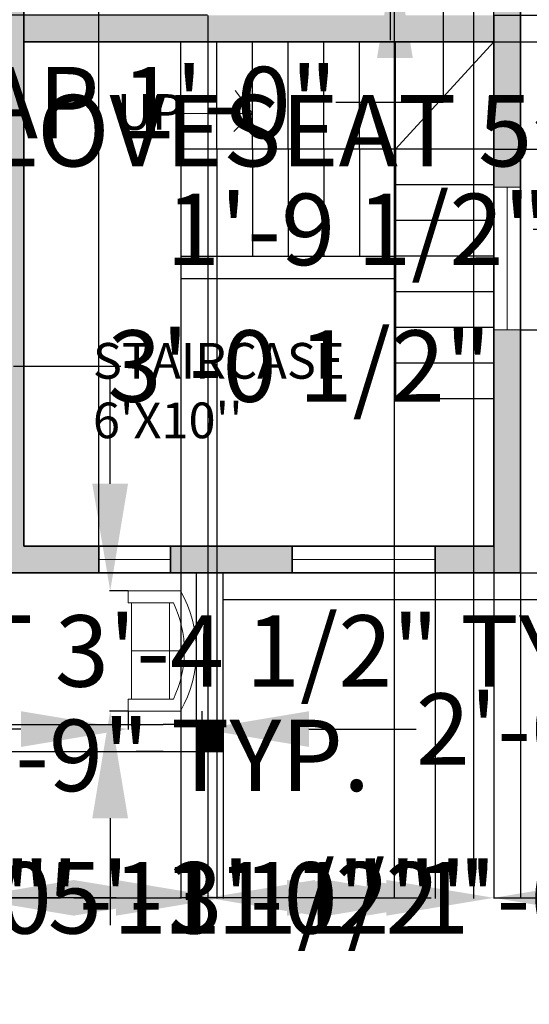
# Model space of a CAD drawing. Units: inches. Extents: x 2838 to 4029, y 1041 to 1915.
# Tile 3 of 16: x 3460 to 3631, y 1046 to 1377. Entities that reach past the tile are written whole.
import ezdxf

# ---------------------------------------------------------------- set-up
doc = ezdxf.new("R2010")
doc.units = ezdxf.units.IN
doc.header["$MEASUREMENT"] = 0
for name, color, linetype, lineweight in [('A-ANNO-DIMS', 2, 'Continuous', 18), ('A-ANNO-SYMB', 2, 'Continuous', 18), ('A-AREA-IDEN', 7, 'Continuous', 18), ('A-COLS', 7, 'Continuous', 35), ('A-FLOR', 7, 'Continuous', 25), ('A-FLOR-STRS', 7, 'Continuous', 25), ('A-FURN', 8, 'Continuous', 18), ('A-GLAZ', 4, 'Continuous', 18), ('A-WALL', 7, 'Continuous', 35), ('A-WALL-PATT', 252, 'Continuous', 13)]:
    doc.layers.add(name, color=color, linetype=linetype, lineweight=lineweight)
doc.styles.get("Standard").update_dxf_attribs({"font": 'arial.ttf'})
doc.dimstyles.get("Standard").update_dxf_attribs({"dimtxt": 24, "dimasz": 36, "dimexe": 0.18, "dimexo": 0.0625, "dimgap": 0.09, "dimtad": 0, "dimtih": 1, "dimtoh": 1, "dimdec": 0, "dimzin": 0, "dimdsep": 46, "dimlunit": 3, "dimtxsty": 'Standard', "dimcen": 0.09, "dimadec": 0, "dimazin": 0, "dimtfac": 1, "dimtdec": 0, "dimtofl": 0, "dimtmove": 0, "dimatfit": 3, "dimfxl": 1, "dimtolj": 1, "dimtzin": 0, "dimarcsym": 0})

# ---------------------------------------------------------------- blocks, each defined once
blk = doc.blocks.new('Sofa - Roundback Loveseat 5 ft.')
for p, q in [((0, -32.44198), (0, -5.99998)), ((-24, -33.99998), (-24, -11.46958)), ((-23.9998, -13.38178), (23.99986, -13.38178)), ((24.00004, -33.99998), (24.00004, -11.46958)), ((-24, -32.44198), (24.00004, -32.44198))]:
    blk.add_line(p, q)
for points in [[(-24, -33.99998), (-30, -33.99998), (-30, -7.99998)], [(30.00004, -7.99998), (30.00004, -33.99998), (24.00004, -33.99998)]]:
    blk.add_lwpolyline(points)
for centre, radius, start, end in [((0, -60.24998), 60.24998, 60.13715, 119.8628), ((0, -61.38438), 55.38444, 64.32083, 115.6792)]:
    blk.add_arc(centre, radius, start, end)
blk = doc.blocks.new('*D17')
at = {"layer": 'A-ANNO-DIMS', "color": 0, "lineweight": -2, "transparency": 16777216}
for p, q in [((3627.79, 1671.3), (3713.18, 1671.3)), ((3713, 1635.3), (3713, 1443.64)), ((3713, 1227.3), (3713, 1418.95)), ((3627.79, 1191.3), (3713.18, 1191.3))]:
    blk.add_line(p, q, dxfattribs=at)
at = {"layer": 'A-ANNO-DIMS', "color": 0, "transparency": 16777216}
for points in [[(3707, 1635.3), (3719, 1635.3), (3713, 1671.3)], [(3707, 1227.3), (3719, 1227.3), (3713, 1191.3)]]:
    blk.add_solid(points, dxfattribs=at)
at = {"layer": 'Defpoints', "color": 0, "transparency": 16777216}
for p in [(3627.73, 1671.3), (3627.73, 1191.3), (3713, 1191.3)]:
    blk.add_point(p, dxfattribs=at)
at = {"layer": 'A-ANNO-DIMS', "color": 0, "transparency": 16777216, "insert": (3713, 1431.3), "char_height": 24, "attachment_point": 5}
blk.add_mtext("\\A1;40'", dxfattribs=at)
blk = doc.blocks.new('WIN-48')
blk.add_line((4.5, 48), (4.5, 0))
blk.add_lwpolyline([(0, 48), (9, 48), (9, 0), (0, 0)], close=True)
blk = doc.blocks.new('WIN-24-VENT')
for p, q in [((24, 9), (24, 0)), ((24, 4.5), (0, 4.5))]:
    blk.add_line(p, q)
blk.add_lwpolyline([(48, 0), (0, 0), (0, 9), (48, 9)])
blk = doc.blocks.new('PORCH-PIER-9X9')
blk.add_lwpolyline([(9, 9), (0, 9), (0, 0), (9, 0)], close=True)
blk = doc.blocks.new('*D29')
at = {"layer": 'A-ANNO-DIMS', "color": 0, "lineweight": -2, "transparency": 16777216}
for p, q in [((3310.15, 1348.85), (3310.15, 1339.73)), ((3370.15, 1348.85), (3370.15, 1339.73)), ((3274.15, 1339.91), (3238.15, 1339.91)), ((3406.15, 1339.91), (3442.15, 1339.91))]:
    blk.add_line(p, q, dxfattribs=at)
at = {"layer": 'A-ANNO-DIMS', "color": 0, "transparency": 16777216}
for points in [[(3274.15, 1345.91), (3274.15, 1333.91), (3310.15, 1339.91)], [(3406.15, 1345.91), (3406.15, 1333.91), (3370.15, 1339.91)]]:
    blk.add_solid(points, dxfattribs=at)
at = {"layer": 'Defpoints', "color": 0, "transparency": 16777216}
for p in [(3310.15, 1348.91), (3370.15, 1348.91), (3370.15, 1339.91)]:
    blk.add_point(p, dxfattribs=at)
at = {"layer": 'A-ANNO-DIMS', "color": 0, "transparency": 16777216, "insert": (3566.77, 1339.91), "char_height": 24, "attachment_point": 5}
blk.add_mtext('\\A1;LOVESEAT 5\'-0"', dxfattribs=at)
blk = doc.blocks.new('*D31')
at = {"layer": 'A-ANNO-DIMS', "color": 0, "lineweight": -2, "transparency": 16777216}
for p, q in [((3489.98, 1221.23), (3489.98, 1257.23)), ((3495.97, 1185.23), (3489.8, 1185.23)), ((3495.97, 1144.84), (3489.8, 1144.84)), ((3489.98, 1108.84), (3489.98, 1072.84))]:
    blk.add_line(p, q, dxfattribs=at)
at = {"layer": 'A-ANNO-DIMS', "color": 0, "transparency": 16777216}
for points in [[(3483.98, 1221.23), (3495.98, 1221.23), (3489.98, 1185.23)], [(3483.98, 1108.84), (3495.98, 1108.84), (3489.98, 1144.84)]]:
    blk.add_solid(points, dxfattribs=at)
at = {"layer": 'Defpoints', "color": 0, "transparency": 16777216}
for p in [(3496.03, 1185.23), (3489.98, 1144.84), (3496.03, 1144.84)]:
    blk.add_point(p, dxfattribs=at)
at = {"layer": 'A-ANNO-DIMS', "color": 0, "transparency": 16777216, "insert": (3489.98, 1165.04), "char_height": 24, "attachment_point": 5}
blk.add_mtext('\\A1;LOVESEAT 3\'-4 1/2" TYP.', dxfattribs=at)
blk = doc.blocks.new('*D32')
at = {"layer": 'A-ANNO-DIMS', "color": 0, "lineweight": -2, "transparency": 16777216}
for p, q in [((3496.03, 1144.78), (3496.03, 1138.61)), ((3520.71, 1144.78), (3520.71, 1138.61)), ((3460.03, 1138.79), (3424.03, 1138.79)), ((3556.71, 1138.79), (3592.71, 1138.79))]:
    blk.add_line(p, q, dxfattribs=at)
at = {"layer": 'A-ANNO-DIMS', "color": 0, "transparency": 16777216}
for points in [[(3460.03, 1144.79), (3460.03, 1132.79), (3496.03, 1138.79)], [(3556.71, 1144.79), (3556.71, 1132.79), (3520.71, 1138.79)]]:
    blk.add_solid(points, dxfattribs=at)
at = {"layer": 'Defpoints', "color": 0, "transparency": 16777216}
for p in [(3496.03, 1144.84), (3520.71, 1144.84), (3520.71, 1138.79)]:
    blk.add_point(p, dxfattribs=at)
at = {"layer": 'A-ANNO-DIMS', "color": 0, "transparency": 16777216, "insert": (3694.12, 1138.79), "char_height": 24, "attachment_point": 5}
blk.add_mtext('\\A1;2\'-0 1/2" TYP.', dxfattribs=at)
blk = doc.blocks.new('*D33')
at = {"layer": 'A-ANNO-DIMS', "color": 0, "lineweight": -2, "transparency": 16777216}
for p, q in [((3601.73, 1469.45), (3601.73, 1505.45)), ((3603.48, 1433.45), (3601.55, 1433.45)), ((3603.48, 1421.37), (3601.55, 1421.37)), ((3601.73, 1385.37), (3601.73, 1349.37)), ((3601.73, 1349.37), (3565.73, 1349.37))]:
    blk.add_line(p, q, dxfattribs=at)
at = {"layer": 'A-ANNO-DIMS', "color": 0, "transparency": 16777216}
for points in [[(3595.73, 1469.45), (3607.73, 1469.45), (3601.73, 1433.45)], [(3595.73, 1385.37), (3607.73, 1385.37), (3601.73, 1421.37)]]:
    blk.add_solid(points, dxfattribs=at)
at = {"layer": 'Defpoints', "color": 0, "transparency": 16777216}
for p in [(3603.54, 1433.45), (3601.73, 1421.37), (3603.54, 1421.37)]:
    blk.add_point(p, dxfattribs=at)
at = {"layer": 'A-ANNO-DIMS', "color": 0, "transparency": 16777216, "insert": (3496.18, 1349.37), "char_height": 24, "attachment_point": 5}
blk.add_mtext('\\A1;TAP 1\'-0"', dxfattribs=at)
blk = doc.blocks.new('*D43')
at = {"layer": 'A-ANNO-DIMS', "color": 0, "lineweight": -2, "transparency": 16777216}
for p, q in [((3231.73, 1129.95), (3195.73, 1129.95)), ((3267.73, 1131.23), (3267.73, 1129.77)), ((3276.73, 1131.23), (3276.73, 1129.77)), ((3312.73, 1129.95), (3348.73, 1129.95))]:
    blk.add_line(p, q, dxfattribs=at)
at = {"layer": 'A-ANNO-DIMS', "color": 0, "transparency": 16777216}
for points in [[(3231.73, 1135.95), (3231.73, 1123.95), (3267.73, 1129.95)], [(3312.73, 1135.95), (3312.73, 1123.95), (3276.73, 1129.95)]]:
    blk.add_solid(points, dxfattribs=at)
at = {"layer": 'Defpoints', "color": 0, "transparency": 16777216}
for p in [(3267.73, 1131.3), (3276.73, 1131.3), (3276.73, 1129.95)]:
    blk.add_point(p, dxfattribs=at)
at = {"layer": 'A-ANNO-DIMS', "color": 0, "transparency": 16777216, "insert": (3465.15, 1129.95), "char_height": 24, "attachment_point": 5}
blk.add_mtext('\\A1;PIER 0\'-9" TYP.', dxfattribs=at)
blk = doc.blocks.new('*D49')
at = {"layer": 'A-ANNO-DIMS', "color": 0, "lineweight": -2, "transparency": 16777216}
for p, q in [((3336.37, 1426.68), (3336.37, 1412.92)), ((3427.37, 1426.68), (3427.37, 1412.92)), ((3372.37, 1413.1), (3391.37, 1413.1)), ((3427.37, 1413.1), (3463.37, 1413.1))]:
    blk.add_line(p, q, dxfattribs=at)
at = {"layer": 'A-ANNO-DIMS', "color": 0, "transparency": 16777216}
for points in [[(3372.37, 1419.1), (3372.37, 1407.1), (3336.37, 1413.1)], [(3391.37, 1419.1), (3391.37, 1407.1), (3427.37, 1413.1)]]:
    blk.add_solid(points, dxfattribs=at)
at = {"layer": 'Defpoints', "color": 0, "transparency": 16777216}
for p in [(3336.37, 1426.75), (3427.37, 1426.75), (3427.37, 1413.1)]:
    blk.add_point(p, dxfattribs=at)
at = {"layer": 'A-ANNO-DIMS', "color": 0, "transparency": 16777216, "insert": (3595.36, 1413.1), "char_height": 24, "attachment_point": 5}
blk.add_mtext('\\A1;DINING SET 7\'-7"', dxfattribs=at)
blk = doc.blocks.new('*D50')
at = {"layer": 'A-ANNO-DIMS', "color": 0, "lineweight": -2, "transparency": 16777216}
for p, q in [((3441.02, 1517.75), (3441.02, 1553.75)), ((3427.44, 1481.75), (3441.2, 1481.75)), ((3427.44, 1426.75), (3441.2, 1426.75)), ((3441.02, 1390.75), (3441.02, 1354.75))]:
    blk.add_line(p, q, dxfattribs=at)
at = {"layer": 'A-ANNO-DIMS', "color": 0, "transparency": 16777216}
for points in [[(3435.02, 1517.75), (3447.02, 1517.75), (3441.02, 1481.75)], [(3435.02, 1390.75), (3447.02, 1390.75), (3441.02, 1426.75)]]:
    blk.add_solid(points, dxfattribs=at)
at = {"layer": 'Defpoints', "color": 0, "transparency": 16777216}
for p in [(3427.37, 1481.75), (3441.02, 1481.75), (3427.37, 1426.75)]:
    blk.add_point(p, dxfattribs=at)
at = {"layer": 'A-ANNO-DIMS', "color": 0, "transparency": 16777216, "insert": (3441.02, 1454.25), "char_height": 24, "attachment_point": 5}
blk.add_mtext('\\A1;4\'-7"', dxfattribs=at)
blk = doc.blocks.new('*D52')
at = {"layer": 'A-ANNO-DIMS', "color": 0, "lineweight": -2, "transparency": 16777216}
for p, q in [((3384.87, 1273.35), (3384.87, 1260.63)), ((3421.54, 1273.35), (3421.54, 1260.63)), ((3348.87, 1260.81), (3312.87, 1260.81)), ((3457.54, 1260.81), (3493.54, 1260.81))]:
    blk.add_line(p, q, dxfattribs=at)
at = {"layer": 'A-ANNO-DIMS', "color": 0, "transparency": 16777216}
for points in [[(3348.87, 1266.81), (3348.87, 1254.81), (3384.87, 1260.81)], [(3457.54, 1266.81), (3457.54, 1254.81), (3421.54, 1260.81)]]:
    blk.add_solid(points, dxfattribs=at)
at = {"layer": 'Defpoints', "color": 0, "transparency": 16777216}
for p in [(3384.87, 1273.41), (3421.54, 1273.41), (3421.54, 1260.81)]:
    blk.add_point(p, dxfattribs=at)
at = {"layer": 'A-ANNO-DIMS', "color": 0, "transparency": 16777216, "insert": (3553.48, 1260.81), "char_height": 24, "attachment_point": 5}
blk.add_mtext('\\A1;3\'-0 1/2"', dxfattribs=at)
blk = doc.blocks.new('*D53')
at = {"layer": 'A-ANNO-DIMS', "color": 0, "lineweight": -2, "transparency": 16777216}
for p, q in [((3583.96, 1508.36), (3583.96, 1544.36)), ((3588.4, 1472.36), (3583.78, 1472.36)), ((3588.4, 1442.36), (3583.78, 1442.36)), ((3583.96, 1406.36), (3583.96, 1370.36))]:
    blk.add_line(p, q, dxfattribs=at)
at = {"layer": 'A-ANNO-DIMS', "color": 0, "transparency": 16777216}
for points in [[(3577.96, 1508.36), (3589.96, 1508.36), (3583.96, 1472.36)], [(3577.96, 1406.36), (3589.96, 1406.36), (3583.96, 1442.36)]]:
    blk.add_solid(points, dxfattribs=at)
at = {"layer": 'Defpoints', "color": 0, "transparency": 16777216}
for p in [(3588.46, 1472.36), (3583.96, 1442.36), (3588.46, 1442.36)]:
    blk.add_point(p, dxfattribs=at)
at = {"layer": 'A-ANNO-DIMS', "color": 0, "transparency": 16777216, "insert": (3583.96, 1457.36), "char_height": 24, "attachment_point": 5}
blk.add_mtext('\\A1;RANGE 2\'-6"', dxfattribs=at)
blk = doc.blocks.new('*D57')
at = {"layer": 'A-ANNO-DIMS', "color": 0, "lineweight": -2, "transparency": 16777216}
for p, q in [((3585.57, 1472.38), (3585.57, 1508.38)), ((3590.9, 1436.38), (3585.39, 1436.38)), ((3590.9, 1400.38), (3585.39, 1400.38)), ((3585.57, 1364.38), (3585.57, 1328.38))]:
    blk.add_line(p, q, dxfattribs=at)
at = {"layer": 'A-ANNO-DIMS', "color": 0, "transparency": 16777216}
for points in [[(3579.57, 1472.38), (3591.57, 1472.38), (3585.57, 1436.38)], [(3579.57, 1364.38), (3591.57, 1364.38), (3585.57, 1400.38)]]:
    blk.add_solid(points, dxfattribs=at)
at = {"layer": 'Defpoints', "color": 0, "transparency": 16777216}
for p in [(3590.97, 1436.38), (3585.57, 1400.38), (3590.97, 1400.38)]:
    blk.add_point(p, dxfattribs=at)
at = {"layer": 'A-ANNO-DIMS', "color": 0, "transparency": 16777216, "insert": (3585.57, 1418.38), "char_height": 24, "attachment_point": 5}
blk.add_mtext('\\A1;DOUBLE SINK 3\'-0"', dxfattribs=at)
blk = doc.blocks.new('*D65')
at = {"layer": 'A-ANNO-DIMS', "color": 0, "lineweight": -2, "transparency": 16777216}
for p, q in [((3267.73, 1131.23), (3267.73, 1081.89)), ((3527.95, 1131.23), (3527.95, 1081.89)), ((3303.73, 1082.07), (3356.32, 1082.07)), ((3491.95, 1082.07), (3439.36, 1082.07))]:
    blk.add_line(p, q, dxfattribs=at)
at = {"layer": 'A-ANNO-DIMS', "color": 0, "transparency": 16777216}
for points in [[(3303.73, 1088.07), (3303.73, 1076.07), (3267.73, 1082.07)], [(3491.95, 1088.07), (3491.95, 1076.07), (3527.95, 1082.07)]]:
    blk.add_solid(points, dxfattribs=at)
at = {"layer": 'Defpoints', "color": 0, "transparency": 16777216}
for p in [(3267.73, 1131.3), (3527.95, 1131.3), (3527.95, 1082.07)]:
    blk.add_point(p, dxfattribs=at)
at = {"layer": 'A-ANNO-DIMS', "color": 0, "transparency": 16777216, "insert": (3397.84, 1082.07), "char_height": 24, "attachment_point": 5}
blk.add_mtext('\\A1;21\'-8"', dxfattribs=at)
blk = doc.blocks.new('*D70')
at = {"layer": 'A-ANNO-DIMS', "color": 0, "lineweight": -2, "transparency": 16777216}
for p, q in [((3329.66, 1113.23), (3329.66, 1081.89)), ((3401.28, 1113.23), (3401.28, 1081.89)), ((3293.66, 1082.07), (3257.66, 1082.07)), ((3437.28, 1082.07), (3473.28, 1082.07))]:
    blk.add_line(p, q, dxfattribs=at)
at = {"layer": 'A-ANNO-DIMS', "color": 0, "transparency": 16777216}
for points in [[(3293.66, 1088.07), (3293.66, 1076.07), (3329.66, 1082.07)], [(3437.28, 1088.07), (3437.28, 1076.07), (3401.28, 1082.07)]]:
    blk.add_solid(points, dxfattribs=at)
at = {"layer": 'Defpoints', "color": 0, "transparency": 16777216}
for p in [(3329.66, 1113.3), (3401.28, 1113.3), (3401.28, 1082.07)]:
    blk.add_point(p, dxfattribs=at)
at = {"layer": 'A-ANNO-DIMS', "color": 0, "transparency": 16777216, "insert": (3542.56, 1082.07), "char_height": 24, "attachment_point": 5}
blk.add_mtext('\\A1;5\'-11 1/2"', dxfattribs=at)
blk = doc.blocks.new('*D71')
at = {"layer": 'A-ANNO-DIMS', "color": 0, "lineweight": -2, "transparency": 16777216}
for p, q in [((3267.73, 1131.23), (3267.73, 1081.89)), ((3329.66, 1113.23), (3329.66, 1081.89)), ((3231.73, 1082.07), (3195.73, 1082.07)), ((3365.66, 1082.07), (3401.66, 1082.07))]:
    blk.add_line(p, q, dxfattribs=at)
at = {"layer": 'A-ANNO-DIMS', "color": 0, "transparency": 16777216}
for points in [[(3231.73, 1088.07), (3231.73, 1076.07), (3267.73, 1082.07)], [(3365.66, 1088.07), (3365.66, 1076.07), (3329.66, 1082.07)]]:
    blk.add_solid(points, dxfattribs=at)
at = {"layer": 'Defpoints', "color": 0, "transparency": 16777216}
for p in [(3267.73, 1131.3), (3329.66, 1113.3), (3329.66, 1082.07)]:
    blk.add_point(p, dxfattribs=at)
at = {"layer": 'A-ANNO-DIMS', "color": 0, "transparency": 16777216, "insert": (3433.65, 1082.07), "char_height": 24, "attachment_point": 5}
blk.add_mtext('\\A1;5\'-2"', dxfattribs=at)
blk = doc.blocks.new('*D73')
at = {"layer": 'A-ANNO-DIMS', "color": 0, "lineweight": -2, "transparency": 16777216}
for p, q in [((3425.038746, 1711.522346), (3389.038746, 1711.522346)), ((3461.038746, 1200.359846), (3461.038746, 1711.702346)), ((3618.731626, 1200.359846), (3618.731626, 1711.702346)), ((3654.731626, 1711.522346), (3690.731626, 1711.522346))]:
    blk.add_line(p, q, dxfattribs=at)
at = {"layer": 'A-ANNO-DIMS', "color": 0, "transparency": 16777216}
for points in [[(3425.038746, 1717.522346), (3425.038746, 1705.522346), (3461.038746, 1711.522346)], [(3654.731626, 1717.522346), (3654.731626, 1705.522346), (3618.731626, 1711.522346)]]:
    blk.add_solid(points, dxfattribs=at)
at = {"layer": 'Defpoints', "color": 0, "transparency": 16777216}
for p in [(3618.731626, 1711.522346), (3461.038746, 1200.297346), (3618.731626, 1200.297346)]:
    blk.add_point(p, dxfattribs=at)
at = {"layer": 'A-ANNO-DIMS', "color": 0, "transparency": 16777216, "insert": (3539.885186, 1711.522346), "char_height": 24, "attachment_point": 5}
blk.add_mtext('\\A1;13\'-1 1/2"', dxfattribs=at)
blk = doc.blocks.new('*D74')
at = {"layer": 'A-ANNO-DIMS', "color": 0, "lineweight": -2, "transparency": 16777216}
for p, q in [((3513.73, 1297.66), (3513.73, 1081.89)), ((3525.73, 1297.66), (3525.73, 1081.89)), ((3477.73, 1082.07), (3441.73, 1082.07)), ((3561.73, 1082.07), (3597.73, 1082.07))]:
    blk.add_line(p, q, dxfattribs=at)
at = {"layer": 'A-ANNO-DIMS', "color": 0, "transparency": 16777216}
for points in [[(3477.73, 1088.07), (3477.73, 1076.07), (3513.73, 1082.07)], [(3561.73, 1088.07), (3561.73, 1076.07), (3525.73, 1082.07)]]:
    blk.add_solid(points, dxfattribs=at)
at = {"layer": 'Defpoints', "color": 0, "transparency": 16777216}
for p in [(3513.73, 1297.73), (3525.73, 1297.73), (3525.73, 1082.07)]:
    blk.add_point(p, dxfattribs=at)
at = {"layer": 'A-ANNO-DIMS', "color": 0, "transparency": 16777216, "insert": (3628.59, 1082.07), "char_height": 24, "attachment_point": 5}
blk.add_mtext('\\A1;1\'-0"', dxfattribs=at)
blk = doc.blocks.new('*D75')
at = {"layer": 'A-ANNO-DIMS', "color": 0, "lineweight": -2, "transparency": 16777216}
for p, q in [((3667.956626, 1405.727214), (3667.956626, 1441.727214)), ((3618.794126, 1369.727214), (3668.136626, 1369.727214)), ((3618.794126, 1333.727214), (3668.136626, 1333.727214)), ((3667.956626, 1297.727214), (3667.956626, 1261.727214))]:
    blk.add_line(p, q, dxfattribs=at)
at = {"layer": 'A-ANNO-DIMS', "color": 0, "transparency": 16777216}
for points in [[(3661.956626, 1405.727214), (3673.956626, 1405.727214), (3667.956626, 1369.727214)], [(3661.956626, 1297.727214), (3673.956626, 1297.727214), (3667.956626, 1333.727214)]]:
    blk.add_solid(points, dxfattribs=at)
at = {"layer": 'Defpoints', "color": 0, "transparency": 16777216}
for p in [(3618.731626, 1369.727214), (3667.956626, 1369.727214), (3618.731626, 1333.727214)]:
    blk.add_point(p, dxfattribs=at)
at = {"layer": 'A-ANNO-DIMS', "color": 0, "transparency": 16777216, "insert": (3667.956626, 1351.727214), "char_height": 24, "attachment_point": 5}
blk.add_mtext('\\A1;3\'-0"', dxfattribs=at)
blk = doc.blocks.new('*D82')
at = {"layer": 'A-ANNO-DIMS', "color": 0, "lineweight": -2, "transparency": 16777216}
for p, q in [((3405.73, 1573.06), (3405.73, 1081.89)), ((3441.73, 1569.23), (3441.73, 1081.89)), ((3369.73, 1082.07), (3333.73, 1082.07)), ((3477.73, 1082.07), (3513.73, 1082.07))]:
    blk.add_line(p, q, dxfattribs=at)
at = {"layer": 'A-ANNO-DIMS', "color": 0, "transparency": 16777216}
for points in [[(3369.73, 1088.07), (3369.73, 1076.07), (3405.73, 1082.07)], [(3477.73, 1088.07), (3477.73, 1076.07), (3441.73, 1082.07)]]:
    blk.add_solid(points, dxfattribs=at)
at = {"layer": 'Defpoints', "color": 0, "transparency": 16777216}
for p in [(3405.73, 1573.12), (3441.73, 1569.3), (3441.73, 1082.07)]:
    blk.add_point(p, dxfattribs=at)
at = {"layer": 'A-ANNO-DIMS', "color": 0, "transparency": 16777216, "insert": (3545.71, 1082.07), "char_height": 24, "attachment_point": 5}
blk.add_mtext('\\A1;3\'-0"', dxfattribs=at)
blk = doc.blocks.new('*D87')
at = {"layer": 'A-ANNO-DIMS', "color": 0, "lineweight": -2, "transparency": 16777216}
for p, q in [((3227.506626, 1497.394218), (3227.506626, 1533.394218)), ((3513.669126, 1461.394218), (3227.326626, 1461.394218)), ((3513.669126, 1425.394218), (3227.326626, 1425.394218)), ((3227.506626, 1389.394218), (3227.506626, 1353.394218))]:
    blk.add_line(p, q, dxfattribs=at)
at = {"layer": 'A-ANNO-DIMS', "color": 0, "transparency": 16777216}
for points in [[(3221.506626, 1497.394218), (3233.506626, 1497.394218), (3227.506626, 1461.394218)], [(3221.506626, 1389.394218), (3233.506626, 1389.394218), (3227.506626, 1425.394218)]]:
    blk.add_solid(points, dxfattribs=at)
at = {"layer": 'Defpoints', "color": 0, "transparency": 16777216}
for p in [(3227.506626, 1461.394218), (3513.731626, 1461.394218), (3513.731626, 1425.394218)]:
    blk.add_point(p, dxfattribs=at)
at = {"layer": 'A-ANNO-DIMS', "color": 0, "transparency": 16777216, "insert": (3227.506626, 1443.394218), "char_height": 24, "attachment_point": 5}
blk.add_mtext('\\A1;3\'-0"', dxfattribs=at)
blk = doc.blocks.new('*D88')
at = {"layer": 'A-ANNO-DIMS', "color": 0, "lineweight": -2, "transparency": 16777216}
for p, q in [((3522.73, 1378.66), (3522.73, 1081.89)), ((3618.73, 1378.66), (3618.73, 1081.89)), ((3558.73, 1082.07), (3582.73, 1082.07)), ((3618.73, 1082.07), (3654.73, 1082.07))]:
    blk.add_line(p, q, dxfattribs=at)
at = {"layer": 'A-ANNO-DIMS', "color": 0, "transparency": 16777216}
for points in [[(3558.73, 1088.07), (3558.73, 1076.07), (3522.73, 1082.07)], [(3582.73, 1088.07), (3582.73, 1076.07), (3618.73, 1082.07)]]:
    blk.add_solid(points, dxfattribs=at)
at = {"layer": 'Defpoints', "color": 0, "transparency": 16777216}
for p in [(3522.73, 1378.73), (3618.73, 1378.73), (3618.73, 1082.07)]:
    blk.add_point(p, dxfattribs=at)
at = {"layer": 'A-ANNO-DIMS', "color": 0, "transparency": 16777216, "insert": (3686.74, 1082.07), "char_height": 24, "attachment_point": 5}
blk.add_mtext('\\A1;8\'-0"', dxfattribs=at)
blk = doc.blocks.new('*D90')
at = {"layer": 'A-ANNO-DIMS', "color": 0, "lineweight": -2, "transparency": 16777216}
for p, q in [((3667.96, 1457.85), (3667.96, 1493.85)), ((3618.79, 1421.85), (3668.14, 1421.85)), ((3618.79, 1378.73), (3668.14, 1378.73)), ((3667.96, 1342.73), (3667.96, 1306.73))]:
    blk.add_line(p, q, dxfattribs=at)
at = {"layer": 'A-ANNO-DIMS', "color": 0, "transparency": 16777216}
for points in [[(3661.96, 1457.85), (3673.96, 1457.85), (3667.96, 1421.85)], [(3661.96, 1342.73), (3673.96, 1342.73), (3667.96, 1378.73)]]:
    blk.add_solid(points, dxfattribs=at)
at = {"layer": 'Defpoints', "color": 0, "transparency": 16777216}
for p in [(3618.73, 1421.85), (3667.96, 1421.85), (3618.73, 1378.73)]:
    blk.add_point(p, dxfattribs=at)
at = {"layer": 'A-ANNO-DIMS', "color": 0, "transparency": 16777216, "insert": (3667.96, 1400.29), "char_height": 24, "attachment_point": 5}
blk.add_mtext('\\A1;3\'-7"', dxfattribs=at)
blk = doc.blocks.new('*D92')
at = {"layer": 'A-ANNO-DIMS', "color": 0, "lineweight": -2, "transparency": 16777216}
for p, q in [((3585.37, 1402), (3585.37, 1081.89)), ((3618.73, 1378.66), (3618.73, 1081.89)), ((3549.37, 1082.07), (3513.37, 1082.07)), ((3654.73, 1082.07), (3690.73, 1082.07))]:
    blk.add_line(p, q, dxfattribs=at)
at = {"layer": 'A-ANNO-DIMS', "color": 0, "transparency": 16777216}
for points in [[(3549.37, 1088.07), (3549.37, 1076.07), (3585.37, 1082.07)], [(3654.73, 1088.07), (3654.73, 1076.07), (3618.73, 1082.07)]]:
    blk.add_solid(points, dxfattribs=at)
at = {"layer": 'Defpoints', "color": 0, "transparency": 16777216}
for p in [(3585.37, 1402.06), (3618.73, 1378.73), (3618.73, 1082.07)]:
    blk.add_point(p, dxfattribs=at)
at = {"layer": 'A-ANNO-DIMS', "color": 0, "transparency": 16777216, "insert": (3750.89, 1082.07), "char_height": 24, "attachment_point": 5}
blk.add_mtext('\\A1;2\'-9 1/2"', dxfattribs=at)
blk = doc.blocks.new('*D93')
at = {"layer": 'A-ANNO-DIMS', "color": 0, "lineweight": -2, "transparency": 16777216}
for p, q in [((3227.51, 1438.06), (3227.51, 1474.06)), ((3227.51, 1474.06), (3263.51, 1474.06)), ((3522.67, 1402.06), (3227.33, 1402.06)), ((3522.67, 1378.73), (3227.33, 1378.73)), ((3227.51, 1342.73), (3227.51, 1306.73))]:
    blk.add_line(p, q, dxfattribs=at)
at = {"layer": 'A-ANNO-DIMS', "color": 0, "transparency": 16777216}
for points in [[(3221.51, 1438.06), (3233.51, 1438.06), (3227.51, 1402.06)], [(3221.51, 1342.73), (3233.51, 1342.73), (3227.51, 1378.73)]]:
    blk.add_solid(points, dxfattribs=at)
at = {"layer": 'Defpoints', "color": 0, "transparency": 16777216}
for p in [(3227.51, 1402.06), (3522.73, 1402.06), (3522.73, 1378.73)]:
    blk.add_point(p, dxfattribs=at)
at = {"layer": 'A-ANNO-DIMS', "color": 0, "transparency": 16777216, "insert": (3331.65, 1474.06), "char_height": 24, "attachment_point": 5}
blk.add_mtext('\\A1;1\'-11 1/2"', dxfattribs=at)
blk = doc.blocks.new('*D98')
at = {"layer": 'A-ANNO-DIMS', "color": 0, "lineweight": -2, "transparency": 16777216}
for p, q in [((3667.96, 1272.94), (3667.96, 1308.94)), ((3667.96, 1308.94), (3703.96, 1308.94)), ((3627.79, 1272.94), (3668.14, 1272.94)), ((3667.96, 1227.3), (3667.96, 1236.94)), ((3627.79, 1191.3), (3668.14, 1191.3))]:
    blk.add_line(p, q, dxfattribs=at)
at = {"layer": 'A-ANNO-DIMS', "color": 0, "transparency": 16777216}
for points in [[(3661.96, 1236.94), (3673.96, 1236.94), (3667.96, 1272.94)], [(3661.96, 1227.3), (3673.96, 1227.3), (3667.96, 1191.3)]]:
    blk.add_solid(points, dxfattribs=at)
at = {"layer": 'Defpoints', "color": 0, "transparency": 16777216}
for p in [(3627.73, 1272.94), (3667.96, 1272.94), (3627.73, 1191.3)]:
    blk.add_point(p, dxfattribs=at)
at = {"layer": 'A-ANNO-DIMS', "color": 0, "transparency": 16777216, "insert": (3763.97, 1308.94), "char_height": 24, "attachment_point": 5}
blk.add_mtext('\\A1;6\'-9 1/2"', dxfattribs=at)
blk = doc.blocks.new('*D99')
at = {"layer": 'A-ANNO-DIMS', "color": 0, "lineweight": -2, "transparency": 16777216}
for p, q in [((3599.07, 1191.23), (3599.07, 1081.89)), ((3627.73, 1191.23), (3627.73, 1081.89)), ((3563.07, 1082.07), (3527.07, 1082.07)), ((3663.73, 1082.07), (3699.73, 1082.07))]:
    blk.add_line(p, q, dxfattribs=at)
at = {"layer": 'A-ANNO-DIMS', "color": 0, "transparency": 16777216}
for points in [[(3563.07, 1088.07), (3563.07, 1076.07), (3599.07, 1082.07)], [(3663.73, 1088.07), (3663.73, 1076.07), (3627.73, 1082.07)]]:
    blk.add_solid(points, dxfattribs=at)
at = {"layer": 'Defpoints', "color": 0, "transparency": 16777216}
for p in [(3599.07, 1191.3), (3627.73, 1191.3), (3627.73, 1082.07)]:
    blk.add_point(p, dxfattribs=at)
at = {"layer": 'A-ANNO-DIMS', "color": 0, "transparency": 16777216, "insert": (3759.89, 1082.07), "char_height": 24, "attachment_point": 5}
blk.add_mtext('\\A1;2\'-4 1/2"', dxfattribs=at)
blk = doc.blocks.new('*D100')
at = {"layer": 'A-ANNO-DIMS', "color": 0, "lineweight": -2, "transparency": 16777216}
for p, q in [((3372.73, 1191.23), (3372.73, 1081.89)), ((3384.45, 1191.23), (3384.45, 1081.89)), ((3336.73, 1082.07), (3300.73, 1082.07)), ((3420.45, 1082.07), (3456.45, 1082.07))]:
    blk.add_line(p, q, dxfattribs=at)
at = {"layer": 'A-ANNO-DIMS', "color": 0, "transparency": 16777216}
for points in [[(3336.73, 1088.07), (3336.73, 1076.07), (3372.73, 1082.07)], [(3420.45, 1088.07), (3420.45, 1076.07), (3384.45, 1082.07)]]:
    blk.add_solid(points, dxfattribs=at)
at = {"layer": 'Defpoints', "color": 0, "transparency": 16777216}
for p in [(3372.73, 1191.3), (3384.45, 1191.3), (3384.45, 1082.07)]:
    blk.add_point(p, dxfattribs=at)
at = {"layer": 'A-ANNO-DIMS', "color": 0, "transparency": 16777216, "insert": (3525.73, 1082.07), "char_height": 24, "attachment_point": 5}
blk.add_mtext('\\A1;0\'-11 1/2"', dxfattribs=at)
blk = doc.blocks.new('*D101')
at = {"layer": 'A-ANNO-DIMS', "color": 0, "lineweight": -2, "transparency": 16777216}
for p, q in [((3425.04, 1711.52), (3389.04, 1711.52)), ((3461.04, 1200.36), (3461.04, 1711.7)), ((3486.18, 1200.36), (3486.18, 1711.7)), ((3522.18, 1711.52), (3558.18, 1711.52))]:
    blk.add_line(p, q, dxfattribs=at)
at = {"layer": 'A-ANNO-DIMS', "color": 0, "transparency": 16777216}
for points in [[(3425.04, 1717.52), (3425.04, 1705.52), (3461.04, 1711.52)], [(3522.18, 1717.52), (3522.18, 1705.52), (3486.18, 1711.52)]]:
    blk.add_solid(points, dxfattribs=at)
at = {"layer": 'Defpoints', "color": 0, "transparency": 16777216}
for p in [(3486.18, 1711.52), (3461.04, 1200.3), (3486.18, 1200.3)]:
    blk.add_point(p, dxfattribs=at)
at = {"layer": 'A-ANNO-DIMS', "color": 0, "transparency": 16777216, "insert": (3590.37, 1711.52), "char_height": 24, "attachment_point": 5}
blk.add_mtext('\\A1;2\'-1"', dxfattribs=at)
blk = doc.blocks.new('*D106')
at = {"layer": 'A-ANNO-DIMS', "color": 0, "lineweight": -2, "transparency": 16777216}
for p, q in [((3611.97, 1401.82), (3611.97, 1081.89)), ((3618.73, 1378.66), (3618.73, 1081.89)), ((3575.97, 1082.07), (3539.97, 1082.07)), ((3654.73, 1082.07), (3690.73, 1082.07))]:
    blk.add_line(p, q, dxfattribs=at)
at = {"layer": 'A-ANNO-DIMS', "color": 0, "transparency": 16777216}
for points in [[(3575.97, 1088.07), (3575.97, 1076.07), (3611.97, 1082.07)], [(3654.73, 1088.07), (3654.73, 1076.07), (3618.73, 1082.07)]]:
    blk.add_solid(points, dxfattribs=at)
at = {"layer": 'Defpoints', "color": 0, "transparency": 16777216}
for p in [(3611.97, 1401.88), (3618.73, 1378.73), (3618.73, 1082.07)]:
    blk.add_point(p, dxfattribs=at)
at = {"layer": 'A-ANNO-DIMS', "color": 0, "transparency": 16777216, "insert": (3722.72, 1082.07), "char_height": 24, "attachment_point": 5}
blk.add_mtext('\\A1;0\'-7"', dxfattribs=at)
blk = doc.blocks.new('*D107')
at = {"layer": 'A-ANNO-DIMS', "color": 0, "lineweight": -2, "transparency": 16777216}
for p, q in [((3667.96, 1436.38), (3667.96, 1472.38)), ((3610.53, 1400.38), (3668.14, 1400.38)), ((3618.79, 1378.73), (3668.14, 1378.73)), ((3667.96, 1342.73), (3667.96, 1306.73)), ((3667.96, 1306.73), (3631.96, 1306.73))]:
    blk.add_line(p, q, dxfattribs=at)
at = {"layer": 'A-ANNO-DIMS', "color": 0, "transparency": 16777216}
for points in [[(3661.96, 1436.38), (3673.96, 1436.38), (3667.96, 1400.38)], [(3661.96, 1342.73), (3673.96, 1342.73), (3667.96, 1378.73)]]:
    blk.add_solid(points, dxfattribs=at)
at = {"layer": 'Defpoints', "color": 0, "transparency": 16777216}
for p in [(3610.47, 1400.38), (3618.73, 1378.73), (3667.96, 1378.73)]:
    blk.add_point(p, dxfattribs=at)
at = {"layer": 'A-ANNO-DIMS', "color": 0, "transparency": 16777216, "insert": (3573.14, 1306.73), "char_height": 24, "attachment_point": 5}
blk.add_mtext('\\A1;1\'-9 1/2"', dxfattribs=at)

msp = doc.modelspace()

# ---------------------------------------------------------------- hatches: boundary and pattern name
at = {"layer": 'A-WALL-PATT'}
h = msp.add_hatch(color=256, dxfattribs=at)
h.dxf.hatch_style = 1
h.paths.add_polyline_path([(3427.52, 1671.3), (3360.91, 1671.3), (3360.91, 1662.3), (3396.73, 1662.3), (3396.73, 1554.39), (3397.12, 1554.39, -0.007312), (3398.53, 1554.41), (3405.73, 1554.41), (3405.73, 1662.3), (3427.52, 1662.3)])
h.paths.add_polyline_path([(3546.42, 1671.3), (3451.52, 1671.3), (3451.52, 1662.3), (3489.73, 1662.3), (3489.73, 1592.86, -0.016107), (3489.73, 1591.9), (3489.73, 1578.3), (3441.73, 1578.3), (3441.73, 1569.3), (3489.73, 1569.3), (3489.73, 1554.41), (3498.73, 1554.41), (3498.73, 1662.3), (3546.42, 1662.3)])
h.paths.add_polyline_path([(3627.73, 1671.3), (3594.42, 1671.3), (3594.42, 1662.3), (3618.73, 1662.3), (3618.73, 1634.03), (3627.73, 1634.03)])
h.paths.add_polyline_path([(3627.73, 1586.03), (3618.73, 1586.03), (3618.73, 1506.39), (3545.12, 1506.39), (3489.73, 1506.39), (3489.73, 1497.39), (3513.73, 1497.39), (3618.73, 1497.39), (3618.73, 1469.85), (3627.73, 1469.85)])
h.paths.add_polyline_path([(3627.73, 1421.85), (3618.73, 1421.85), (3618.73, 1378.73), (3522.73, 1378.73), (3513.73, 1378.73), (3461.04, 1378.73), (3461.04, 1369.73), (3513.73, 1369.73), (3618.73, 1369.73), (3618.73, 1320.94), (3627.73, 1320.94)])
h.paths.add_polyline_path([(3627.73, 1272.94), (3618.73, 1272.94), (3618.73, 1200.3), (3599.07, 1200.3), (3599.07, 1191.3), (3627.73, 1191.3)])
h.paths.add_polyline_path([(3551.07, 1200.3), (3510.18, 1200.3), (3510.18, 1191.3), (3551.07, 1191.3)])
h.paths.add_polyline_path([(3486.18, 1200.3), (3461.04, 1200.3), (3461.04, 1398.25), (3454.63, 1398.25), (3454.63, 1200.3), (3432.45, 1200.3), (3432.45, 1191.3), (3486.18, 1191.3)])
h.paths.add_polyline_path([(3300.73, 1200.3), (3276.73, 1200.3), (3276.73, 1391.57), (3331.05, 1391.57), (3331.05, 1400.57), (3276.73, 1400.57), (3276.73, 1432.17), (3267.73, 1432.17), (3267.73, 1191.3), (3300.73, 1191.3)])
h = msp.add_hatch(dxfattribs=at)
h.set_pattern_fill('ANSI31', color=256)
h.paths.add_polyline_path([(3527.95, 1140.3), (3518.95, 1140.3), (3518.95, 1131.3), (3527.95, 1131.3)])

# ---------------------------------------------------------------- linework, layer by layer
at = {"layer": 'A-ANNO-SYMB'}
for p, q in [((3537.73, 1345.69), (3531.89, 1353.37)), ((3531.89, 1353.37), (3537.73, 1345.69)), ((3513.73, 1345.69), (3537.73, 1345.69)), ((3537.73, 1345.69), (3531.48, 1339.66))]:
    msp.add_line(p, q, dxfattribs=at)
at = {"layer": 'A-FLOR'}
for p, q in [((3518.95, 1140.3), (3518.95, 1191.3)), ((3527.95, 1132.75), (3527.95, 1191.3)), ((3276.73, 1140.3), (3498.72, 1140.3)), ((3518.95, 1140.3), (3507.72, 1140.3)), ((3527.95, 1131.3), (3527.95, 1132.75)), ((3267.73, 1131.3), (3507.72, 1131.3)), ((3507.72, 1131.3), (3527.95, 1131.3))]:
    msp.add_line(p, q, dxfattribs=at)
for points in [[(3527.95, 1182.3), (3636.73, 1182.3), (3636.73, 1680.3), (3258.73, 1680.3), (3258.73, 1182.3), (3267.73, 1182.3)], [(3498.72, 1140.3), (3507.72, 1140.3)], [(3507.72, 1131.3), (3498.72, 1131.3)]]:
    msp.add_lwpolyline(points, dxfattribs=at)
at = {"layer": 'A-FLOR-STRS'}
for p, q in [((3513.73, 1333.73), (3513.73, 1369.73)), ((3525.73, 1333.73), (3525.73, 1369.73)), ((3537.73, 1333.73), (3537.73, 1369.73)), ((3549.73, 1333.73), (3549.73, 1369.73)), ((3561.73, 1333.73), (3561.73, 1369.73)), ((3573.73, 1333.73), (3573.73, 1369.73)), ((3585.73, 1333.73), (3585.73, 1369.73)), ((3618.73, 1369.73), (3585.73, 1333.73)), ((3618.73, 1333.73), (3513.73, 1333.73)), ((3513.73, 1333.73), (3513.73, 1297.73)), ((3525.73, 1333.73), (3525.73, 1297.73)), ((3537.73, 1333.73), (3537.73, 1297.73)), ((3549.73, 1333.73), (3549.73, 1297.73)), ((3561.73, 1333.73), (3561.73, 1297.73)), ((3573.73, 1333.73), (3573.73, 1297.73)), ((3585.73, 1333.73), (3585.73, 1249.73)), ((3585.73, 1333.73), (3585.73, 1297.73)), ((3618.73, 1321.73), (3585.73, 1321.73)), ((3618.73, 1309.73), (3585.73, 1309.73)), ((3513.73, 1297.73), (3585.73, 1297.73)), ((3513.73, 1297.73), (3513.73, 1290.21)), ((3618.73, 1297.73), (3585.73, 1297.73)), ((3513.73, 1290.21), (3585.73, 1290.21)), ((3618.73, 1285.73), (3585.73, 1285.73)), ((3618.73, 1273.73), (3585.73, 1273.73)), ((3618.73, 1261.73), (3585.73, 1261.73)), ((3618.73, 1249.73), (3585.73, 1249.73))]:
    msp.add_line(p, q, dxfattribs=at)
at = {"layer": 'A-WALL'}
for p, q in [((3627.73, 1191.3), (3627.73, 1671.3)), ((3627.73, 1320.94), (3627.73, 1421.85)), ((3461.04, 1200.3), (3461.04, 1398.25)), ((3513.73, 1369.73), (3461.04, 1369.73)), ((3618.73, 1369.73), (3513.73, 1369.73)), ((3618.73, 1200.3), (3618.73, 1369.73)), ((3627.73, 1272.94), (3627.73, 1320.94)), ((3627.73, 1191.3), (3627.73, 1272.94)), ((3461.04, 1200.3), (3618.73, 1200.3)), ((3486.18, 1191.3), (3486.18, 1200.3)), ((3486.18, 1200.3), (3510.18, 1200.3)), ((3510.18, 1200.3), (3510.18, 1191.3)), ((3551.07, 1191.3), (3551.07, 1200.3)), ((3551.07, 1200.3), (3599.07, 1200.3)), ((3599.07, 1200.3), (3599.07, 1191.3)), ((3432.45, 1191.3), (3486.18, 1191.3)), ((3510.18, 1191.3), (3551.07, 1191.3)), ((3599.07, 1191.3), (3627.73, 1191.3))]:
    msp.add_line(p, q, dxfattribs=at)
msp.add_lwpolyline([(3372.73, 1191.3), (3627.73, 1191.3), (3627.73, 1671.3), (3267.73, 1671.3), (3267.73, 1191.3), (3300.73, 1191.3)], dxfattribs=at)

# ---------------------------------------------------------------- block references
at = {"layer": 'A-COLS', "rotation": 90.00000000000242}
msp.add_blockref('PORCH-PIER-9X9', (3527.95, 1131.3), dxfattribs=at)
at = {"layer": 'A-FURN', "xscale": 0.6730714582278688, "yscale": 0.6730714582278688, "zscale": 0.6730714582278688, "rotation": 270}
msp.add_blockref('Sofa - Roundback Loveseat 5 ft.', (3518.92, 1165.04), dxfattribs=at)
at = {"layer": 'A-GLAZ'}
for name, p in [('WIN-48', (3618.73, 1272.94)), ('WIN-24-VENT', (3486.18, 1191.3))]:
    msp.add_blockref(name, p, dxfattribs=at)
at = {"layer": 'A-GLAZ', "rotation": 269.9999999999991}
msp.add_blockref('WIN-48', (3551.07, 1200.3), dxfattribs=at)

# ---------------------------------------------------------------- texts
at = {"layer": 'A-ANNO-SYMB', "insert": (3492.23, 1352.2), "char_height": 12, "attachment_point": 1}
msp.add_mtext_dynamic_manual_height_columns('UP', width=14.7812, gutter_width=1, heights=[0], dxfattribs=at)
at = {"layer": 'A-AREA-IDEN', "insert": (3484.18, 1268.55), "char_height": 12, "attachment_point": 1}
msp.add_mtext_dynamic_manual_height_columns("STAIRCASE\\P6'X10''", width=64.6015, gutter_width=1, heights=[0], dxfattribs=at)

# ---------------------------------------------------------------- dimensions: what is measured, and where the dimension line sits
at = {"layer": 'A-ANNO-DIMS'}
for base, p1, p2, picture, middle in [((3618.73, 1711.52), (3461.04, 1200.3), (3618.73, 1200.3), '*D73', (3539.89, 1711.52)), ((3486.18, 1711.52), (3461.04, 1200.3), (3486.18, 1200.3), '*D101', (3590.37, 1711.52)), ((3441.73, 1082.07), (3405.73, 1573.12), (3441.73, 1569.3), '*D82', (3545.71, 1082.07)), ((3618.73, 1082.07), (3585.37, 1402.06), (3618.73, 1378.73), '*D92', (3750.89, 1082.07)), ((3618.73, 1082.07), (3611.97, 1401.88), (3618.73, 1378.73), '*D106', (3722.72, 1082.07)), ((3618.73, 1082.07), (3522.73, 1378.73), (3618.73, 1378.73), '*D88', (3686.74, 1082.07)), ((3525.73, 1082.07), (3513.73, 1297.73), (3525.73, 1297.73), '*D74', (3628.59, 1082.07)), ((3421.54, 1260.81), (3384.87, 1273.41), (3421.54, 1273.41), '*D52', (3553.48, 1260.81)), ((3384.45, 1082.07), (3372.73, 1191.3), (3384.45, 1191.3), '*D100', (3525.73, 1082.07)), ((3627.73, 1082.07), (3599.07, 1191.3), (3627.73, 1191.3), '*D99', (3759.89, 1082.07)), ((3329.66, 1082.07), (3267.73, 1131.3), (3329.66, 1113.3), '*D71', (3433.65, 1082.07)), ((3527.95, 1082.07), (3267.73, 1131.3), (3527.95, 1131.3), '*D65', (3397.84, 1082.07)), ((3401.28, 1082.07), (3329.66, 1113.3), (3401.28, 1113.3), '*D70', (3542.56, 1082.07))]:
    dim = msp.add_linear_dim(base=base, p1=p1, p2=p2, dimstyle='Standard', override={"dimdec": 1, "dimlfac": 1, "dimrnd": 0, "dimzin": 1, "dimdsep": 46, "dimlunit": 4, "dimfrac": 2}, dxfattribs=at)
    dim.commit()
    dim.dimension.update_dxf_attribs({"geometry": picture, "text_midpoint": middle})
for base, p1, p2, override, picture, middle in [((3713, 1191.3), (3627.73, 1671.3), (3627.73, 1191.3), {"dimclrd": 0, "dimclre": 0, "dimclrt": 0}, '*D17', (3713, 1431.3)), ((3441.02, 1481.75), (3427.37, 1426.75), (3427.37, 1481.75), {"dimdec": 1, "dimlfac": 1, "dimrnd": 0, "dimzin": 1, "dimdsep": 46, "dimlunit": 4, "dimfrac": 2}, '*D50', (3441.02, 1454.25)), ((3227.51, 1461.39), (3513.73, 1425.39), (3513.73, 1461.39), {"dimdec": 1, "dimlfac": 1, "dimrnd": 0, "dimzin": 1, "dimdsep": 46, "dimlunit": 4, "dimfrac": 2}, '*D87', (3227.51, 1443.39)), ((3227.51, 1402.06), (3522.73, 1378.73), (3522.73, 1402.06), {"dimdec": 1, "dimlfac": 1, "dimrnd": 0, "dimzin": 1, "dimdsep": 46, "dimlunit": 4, "dimfrac": 2}, '*D93', (3331.65, 1474.06)), ((3667.96, 1421.85), (3618.73, 1378.73), (3618.73, 1421.85), {"dimdec": 1, "dimlfac": 1, "dimrnd": 0, "dimzin": 1, "dimdsep": 46, "dimlunit": 4, "dimfrac": 2}, '*D90', (3667.96, 1400.29)), ((3667.9566, 1378.7272), (3610.4672, 1400.3841), (3618.7316, 1378.7272), {"dimdec": 1, "dimlfac": 1, "dimrnd": 0, "dimzin": 1, "dimdsep": 46, "dimlunit": 4, "dimfrac": 2}, '*D107', (3573.1354, 1306.7272)), ((3667.96, 1369.73), (3618.73, 1333.73), (3618.73, 1369.73), {"dimdec": 1, "dimlfac": 1, "dimrnd": 0, "dimzin": 1, "dimdsep": 46, "dimlunit": 4, "dimfrac": 2}, '*D75', (3667.96, 1351.73)), ((3667.96, 1272.94), (3627.73, 1191.3), (3627.73, 1272.94), {"dimdec": 1, "dimlfac": 1, "dimrnd": 0, "dimzin": 1, "dimdsep": 46, "dimlunit": 4, "dimfrac": 2}, '*D98', (3763.97, 1308.94))]:
    dim = msp.add_linear_dim(base=base, p1=p1, p2=p2, angle=90, dimstyle='Standard', override=override, dxfattribs=at)
    dim.commit()
    dim.dimension.update_dxf_attribs({"geometry": picture, "text_midpoint": middle})
for base, p1, p2, text, picture, middle in [((3583.96, 1442.36), (3588.46, 1472.36), (3588.46, 1442.36), 'RANGE <>', '*D53', (3583.96, 1457.36)), ((3585.57, 1400.38), (3590.97, 1436.38), (3590.97, 1400.38), 'DOUBLE SINK <>', '*D57', (3585.57, 1418.38)), ((3601.73, 1421.37), (3603.54, 1433.45), (3603.54, 1421.37), 'TAP <>', '*D33', (3496.18, 1349.37)), ((3489.98, 1144.84), (3496.03, 1185.23), (3496.03, 1144.84), 'LOVESEAT <> TYP.', '*D31', (3489.98, 1165.04))]:
    dim = msp.add_linear_dim(base=base, p1=p1, p2=p2, angle=270, text=text, dimstyle='Standard', override={"dimdec": 1, "dimlfac": 1, "dimrnd": 0, "dimzin": 1, "dimdsep": 46, "dimlunit": 4, "dimfrac": 2}, dxfattribs=at)
    dim.commit()
    dim.dimension.update_dxf_attribs({"geometry": picture, "text_midpoint": middle})
for base, p1, p2, text, picture, middle in [((3427.37, 1413.1), (3336.37, 1426.75), (3427.37, 1426.75), 'DINING SET <>', '*D49', (3595.36, 1413.1)), ((3370.15, 1339.91), (3310.15, 1348.91), (3370.15, 1348.91), 'LOVESEAT <>', '*D29', (3566.77, 1339.91)), ((3520.71, 1138.79), (3496.03, 1144.84), (3520.71, 1144.84), '<> TYP.', '*D32', (3694.12, 1138.79)), ((3276.73, 1129.95), (3267.73, 1131.3), (3276.73, 1131.3), 'PIER <> TYP.', '*D43', (3465.15, 1129.95))]:
    dim = msp.add_linear_dim(base=base, p1=p1, p2=p2, text=text, dimstyle='Standard', override={"dimdec": 1, "dimlfac": 1, "dimrnd": 0, "dimzin": 1, "dimdsep": 46, "dimlunit": 4, "dimfrac": 2}, dxfattribs=at)
    dim.commit()
    dim.dimension.update_dxf_attribs({"geometry": picture, "text_midpoint": middle})

doc.saveas('drawing.dxf')
